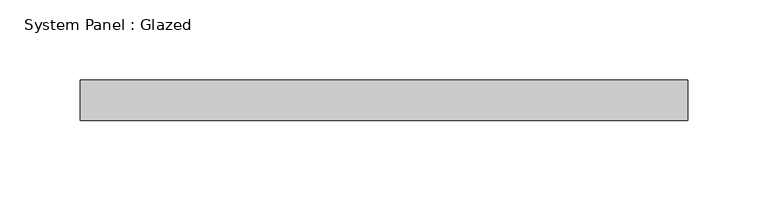
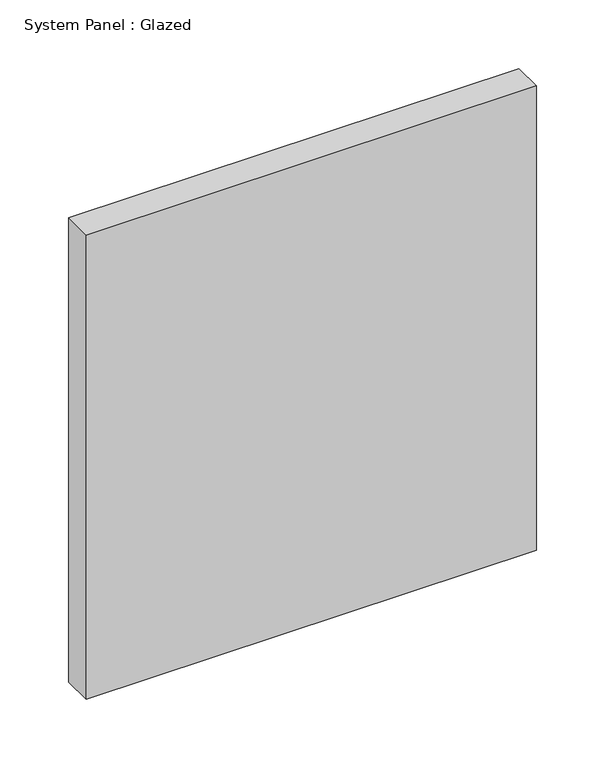
"""IFC4 building model written with IfcOpenShell, lengths in millimetres: plate geometry, System Panel : Glazed."""

from ifc_helpers import new_model, si_unit, origin, origin_with_axes, place, context, project, spatial, polyline, outline, extrude, source, transform, mapped, element, save


def system_panel_glazed_eeed78fb(model_context):
    return source(origin(), model_context, "Body", "SweptSolid", [
        extrude(outline(polyline([(189.4416667, 19.05), (-189.4416667, 19.05), (-189.4416667, 44.45), (189.4416667, 44.45), (189.4416667, 19.05)])), origin_with_axes(), (0.0, 0.0, 1.0), 412.75),
    ])


if __name__ == "__main__":
    model = new_model("IFC4")
    model_context = context("Model", 3, world=origin())
    ifc_project = project(units=[si_unit("LENGTHUNIT", "METRE", prefix="MILLI")], contexts=[model_context])
    site = spatial("IfcSite", under=ifc_project)
    building = spatial("IfcBuilding", under=site)
    placement = place(None, origin())
    system_panel_glazed_shape = system_panel_glazed_eeed78fb(model_context)
    element("IfcPlate", 1, ObjectType="System Panel : Glazed", at=placement, inside=building, context=model_context, shape_type="MappedRepresentation", body=[
        mapped(system_panel_glazed_shape, transform((0.0, 0.0, 0.0), x_axis=(1.0, 0.0, 0.0), y_axis=(0.0, 1.0, 0.0), z_axis=(0.0, 0.0, 1.0))),
    ])
    save(model, "model.ifc")

# Revit data of these elements
# Type "System Panel : Glazed"
#   Construction Type Id = "GSP4R"
#   Analytic Construction = "1/8 in Pilkington single glazing"
#   Visual Light Transmittance = 0.9
#   Solar Heat Gain Coefficient = 0.86
#   Heat Transfer Coefficient (U) = 1.18115 BTU/(h·ft²·°F)
#   Define Thermal Properties by = 1
# Element 1 (IfcPlate, "System Panel : Glazed")
#   Materials on its faces: "Glass"
# Materials
#   "Glass": class "Glass", colour RGB 0 128 192, transparency 0.75, Description = "Soda Lime Glass", Cost = 0
